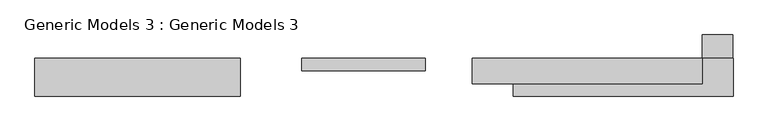
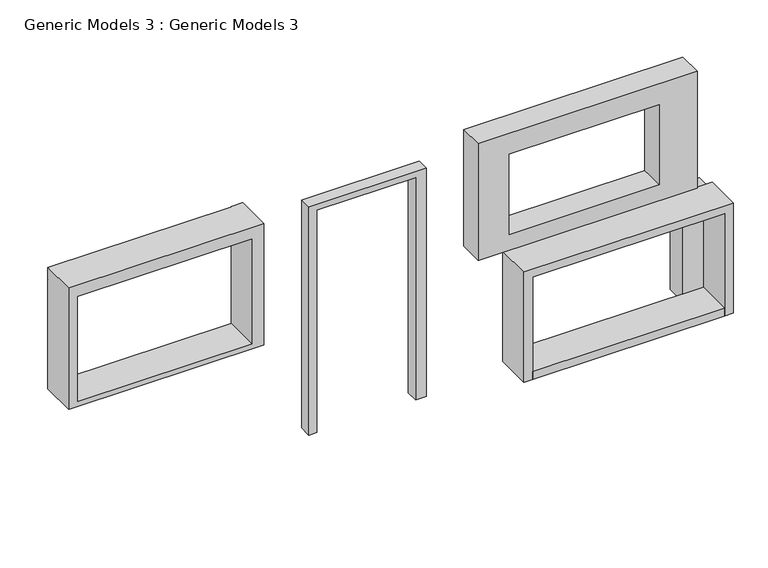
"""IFC4 building model written with IfcOpenShell, lengths in millimetres: proxy geometry, Generic Models 3 : Generic Models 3."""

from ifc_helpers import new_model, si_unit, frame, origin, origin_with_axes, place, context, project, spatial, polyline, outline, extrude, faceted_brep, source, transform, mapped, element, save


def generic_models_3_generic_models_3_82c5f115(model_context):
    return source(origin(), model_context, "Body", "SolidModel", [
        extrude(outline(polyline([(6400.8, -3625.114323), (6400.8, -9034.7947562), (3352.8, -9034.7947562), (3352.8, -3625.114323), (6400.8, -3625.114323)]), holes=[polyline([(5862.3849303, -4567.2344381), (3764.5724927, -4567.2344381), (3764.5724927, -8266.2551029), (5862.3849303, -8266.2551029), (5862.3849303, -4567.2344381)])]), frame((0.0, -14463.7538163, 0.0), z_axis=(0.0, 1.0, 0.0), x_axis=(0.0, 0.0, 1.0)), (0.0, 0.0, 1.0), 609.6),
        extrude(outline(polyline([(2880.6848502, -2901.214323), (2880.6848502, -8072.8951638), (0.0, -8072.8951638), (0.0, -7854.214323), (2677.4848502, -7854.214323), (2677.4848502, -3113.2272536), (0.0, -3113.2272536), (0.0, -2901.214323), (2880.6848502, -2901.214323)])), frame((0.0, -14748.2931134, 0.0), z_axis=(0.0, 1.0, 0.0), x_axis=(0.0, 0.0, 1.0)), (0.0, 0.0, 1.0), 894.1392971),
        extrude(outline(polyline([(-3113.2272536, -14748.2931134), (-7854.214323, -14748.2931134), (-7854.214323, -13854.1538163), (-3113.2272536, -13854.1538163), (-3113.2272536, -14748.2931134)])), origin_with_axes(), (0.0, 0.0, 1.0), 207.9039867),
        extrude(outline(polyline([(-2907.0008035, -13854.1538163), (-3625.114323, -13854.1538163), (-3625.114323, -13310.467207), (-2907.0008035, -13310.467207), (-2907.0008035, -13854.1538163)])), origin_with_axes(), (0.0, 0.0, 1.0), 2677.4848502),
        extrude(outline(polyline([(0.0, -13042.1380521), (0.0, -12845.314323), (5811.5849303, -12845.314323), (5811.5849303, -10406.914323), (0.0, -10406.914323), (0.0, -10145.5548754), (5963.9849303, -10145.5548754), (5963.9849303, -13042.1380521), (0.0, -13042.1380521)])), frame((0.0, -14158.9538163, 0.0), z_axis=(0.0, 1.0, 0.0), x_axis=(0.0, 0.0, 1.0)), (0.0, 0.0, 1.0), 304.8),
        faceted_brep([(-19322.314323, -14748.2931134, 3225.8), (-14496.314323, -14748.2931134, 3225.8), (-14496.314323, -14748.2931134, 6400.8), (-19322.314323, -14748.2931134, 6400.8), (-19093.714323, -14748.2931134, 3352.8), (-19093.714323, -14748.2931134, 6096.0), (-14788.414323, -14748.2931134, 6096.0), (-14788.414323, -14748.2931134, 3352.8), (-19322.314323, -13854.1538163, 3352.8), (-19322.314323, -13854.1538163, 6096.0), (-19093.714323, -13854.1538163, 6096.0), (-19093.714323, -13854.1538163, 3352.8), (-19093.714323, -13864.3466243, 3352.8), (-19322.314323, -13864.3466243, 3352.8), (-19093.714323, -13864.3466243, 6096.0), (-19322.314323, -13864.3466243, 6096.0), (-19322.314323, -13864.3466243, 3225.8), (-19322.314323, -13864.3466243, 6400.8), (-14496.314323, -13864.3466243, 3352.8), (-14496.314323, -13864.3466243, 3225.8), (-14788.414323, -13864.3466243, 3352.8), (-14496.314323, -13854.1538163, 3352.8), (-14496.314323, -13854.1538163, 6400.8), (-14788.414323, -13854.1538163, 3352.8), (-14788.414323, -13854.1538163, 6400.8), (-14788.414323, -13864.3466243, 6400.8), (-14788.414323, -13864.3466243, 6096.0)], [[[0, 1, 2, 3], [4, 5, 6, 7]], [[8, 9, 10, 11]], [[8, 11, 12, 13]], [[5, 4, 12, 11, 10, 14]], [[10, 9, 15, 14]], [[9, 8, 13, 16, 0, 3, 17, 15]], [[18, 19, 16, 13, 12, 20]], [[12, 4, 7, 20]], [[1, 0, 16, 19]], [[19, 18, 21, 22, 2, 1]], [[22, 21, 23, 24]], [[22, 24, 25, 17, 3, 2]], [[24, 23, 20, 7, 6, 26, 25]], [[23, 21, 18, 20]], [[15, 17, 25, 26, 14]], [[6, 5, 14, 26]]]),
    ])


if __name__ == "__main__":
    model = new_model("IFC4")
    model_context = context("Model", 3, world=origin())
    ifc_project = project(units=[si_unit("LENGTHUNIT", "METRE", prefix="MILLI")], contexts=[model_context])
    site = spatial("IfcSite", under=ifc_project)
    building = spatial("IfcBuilding", under=site)
    placement = place(None, origin())
    generic_models_3_generic_models_3_shape = generic_models_3_generic_models_3_82c5f115(model_context)
    element("IfcBuildingElementProxy", 1, Name="Generic Models 3 : Generic Models 3", ObjectType="Generic Models 3 : Generic Models 3", at=placement, inside=building, context=model_context, shape_type="MappedRepresentation", body=[
        mapped(generic_models_3_generic_models_3_shape, transform((0.0, 0.0, 0.0), x_axis=(1.0, 0.0, 0.0), y_axis=(0.0, 1.0, 0.0), z_axis=(0.0, 0.0, 1.0))),
    ])
    save(model, "model.ifc")
